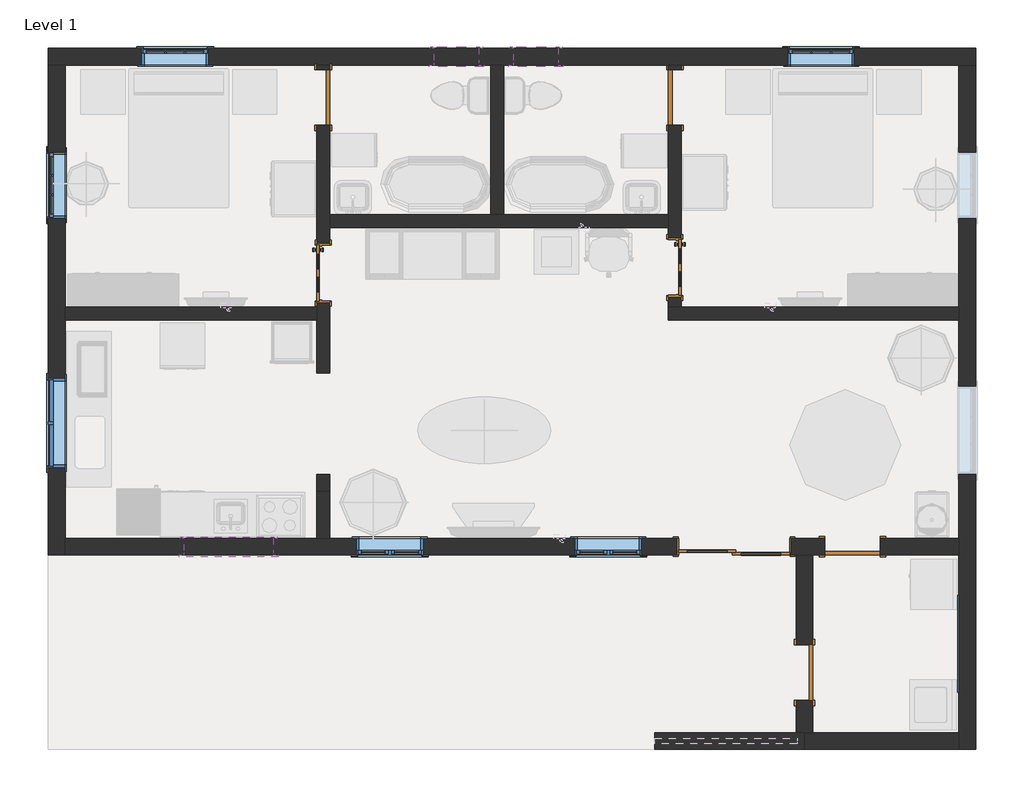
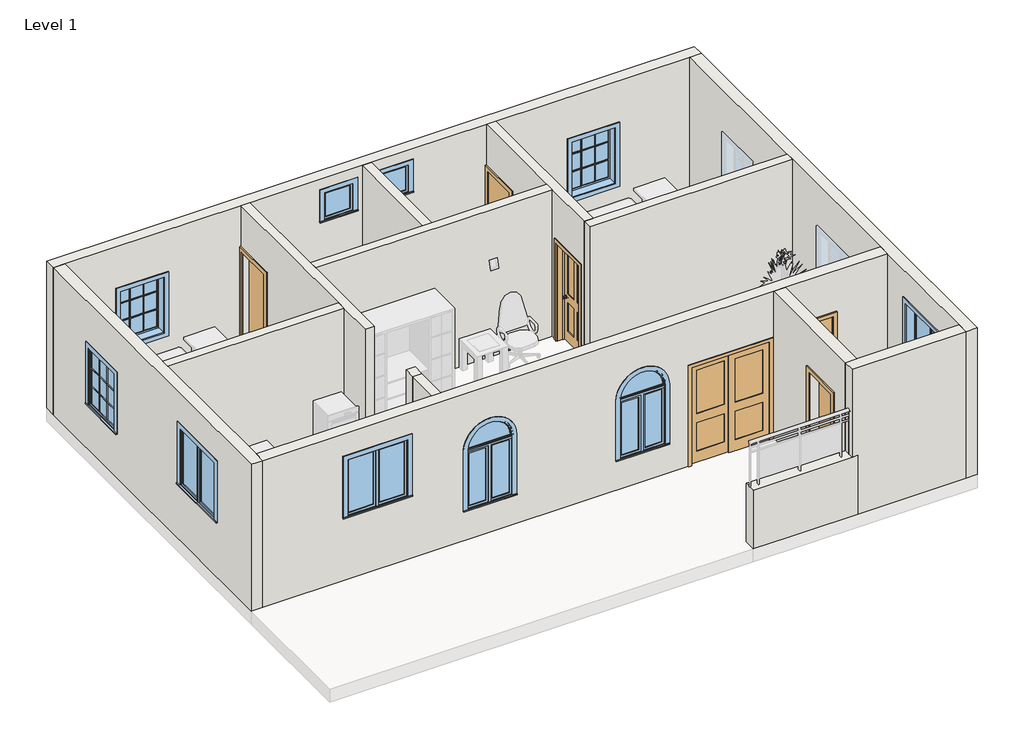
# One storey, part 1 of 2: 15 walls, 10 windows, 7 doors.
"""IFC4 building model written with IfcOpenShell, lengths in millimetres."""

from ifc_helpers import new_model, si_unit, frame, origin, origin_with_axes, place, context, project, spatial, polyline, circle_curve, outline, extrude, faceted_brep, transform, mapped, element, save
from ifc_brep_helpers import plane_surface, revolved_surface, advanced_brep
from components import door_61c74ce0, door_86658926, door_b97b09b3, door_b1104dde, door_0af0cdd0, door_bb98abfd, window_ae0d0e3f, window_642cfea4, window_534dcd48, window_3ed046d9

model = new_model("IFC4")

# Units and contexts
model_context = context("Model", 3, world=origin())
ifc_project = project(units=[si_unit("LENGTHUNIT", "METRE", prefix="MILLI")], contexts=[model_context])

# Site, building, storey
site = spatial("IfcSite", under=ifc_project)
building = spatial("IfcBuilding", under=site)
storey = spatial("IfcBuildingStorey", under=building, Name="Level 1", Elevation=0.0)

# Doors
placement = place(None, origin())
door_shape = door_61c74ce0(model_context)
element("IfcDoor", 1, ObjectType="Door-Interior-Double-Sliding-2_Panel-Wood : 60\" x 80\"", at=placement, inside=storey, context=model_context, shape_type="MappedRepresentation", body=[
    mapped(door_shape, transform((-1370.6447551, 6722.1799175, 0.0), x_axis=(-1.0, 0.0, 0.0), y_axis=(0.0, -1.0, 0.0), z_axis=(0.0, 0.0, 1.0))),
])
door_2_shape = door_86658926(model_context)
element("IfcDoor", 2, ObjectType="Door-Interior-Single-4_Panel-Wood : 30\" x 80\"", at=placement, inside=storey, context=model_context, shape_type="MappedRepresentation", body=[
    mapped(door_2_shape, transform((-7012.6197551, 10484.5549175, 0.0), x_axis=(0.0, -1.0, 0.0), y_axis=(1.0, 0.0, 0.0), z_axis=(0.0, 0.0, 1.0))),
])
door_3_shape = door_b97b09b3(model_context)
element("IfcDoor", 3, ObjectType="Door-Interior-Single-4_Panel-Wood : 30\" x 80\"", at=placement, inside=storey, context=model_context, shape_type="MappedRepresentation", body=[
    mapped(door_3_shape, transform((-2180.2697551, 10560.7549175, 0.0), x_axis=(0.0, -1.0, 0.0), y_axis=(1.0, 0.0, 0.0), z_axis=(0.0, 0.0, 1.0))),
])
door_4_shape = door_b1104dde(model_context)
element("IfcDoor", 4, ObjectType="Single-Flush : 30\" x 84\"", at=placement, inside=storey, context=model_context, shape_type="MappedRepresentation", body=[
    mapped(door_4_shape, transform((-7009.4447551, 12897.5549175, 0.0), x_axis=(0.0, 1.0, 0.0), y_axis=(-1.0, 0.0, 0.0), z_axis=(0.0, 0.0, 1.0))),
])
door_5_shape = door_0af0cdd0(model_context)
element("IfcDoor", 5, ObjectType="Single-Flush : 30\" x 84\"", at=placement, inside=storey, context=model_context, shape_type="MappedRepresentation", body=[
    mapped(door_5_shape, transform((-2183.4447551, 12897.5549175, 0.0), x_axis=(0.0, 1.0, 0.0), y_axis=(-1.0, 0.0, 0.0), z_axis=(0.0, 0.0, 1.0))),
])
door_6_shape = door_bb98abfd(model_context)
element("IfcDoor", 6, ObjectType="Single-Flush : 30\" x 84\"", at=placement, inside=storey, context=model_context, shape_type="MappedRepresentation", body=[
    mapped(door_6_shape, transform((254.9552449, 6725.3549175, 0.0), x_axis=(-1.0, 0.0, 0.0), y_axis=(0.0, -1.0, 0.0), z_axis=(0.0, 0.0, 1.0))),
])
element("IfcDoor", 7, ObjectType="Single-Flush : 30\" x 84\"", at=placement, inside=storey, context=model_context, shape_type="MappedRepresentation", body=[
    mapped(door_6_shape, transform((-405.4447551, 4998.1549175, 0.0), x_axis=(0.0, -1.0, 0.0), y_axis=(1.0, 0.0, 0.0), z_axis=(0.0, 0.0, 1.0))),
])

# Walls
element("IfcWall", 8, ObjectType="Generic - 8\"", at=placement, inside=storey, context=model_context, shape_type="Brep", body=[
    faceted_brep([(-10781.3447551, 13342.0549175, 0.0), (-10552.7447551, 13342.0549175, 0.0), (-7098.3447551, 13342.0549175, 0.0), (-6920.5447551, 13342.0549175, 0.0), (-4710.7447551, 13342.0549175, 0.0), (-4532.9447551, 13342.0549175, 0.0), (-2272.3447551, 13342.0549175, 0.0), (-2094.5447551, 13342.0549175, 0.0), (1715.4552449, 13342.0549175, 0.0), (1944.0552449, 13342.0549175, 0.0), (1944.0552449, 13342.0549175, 3048.0), (1715.4552449, 13342.0549175, 3048.0), (-2094.5447551, 13342.0549175, 3048.0), (-2272.3447551, 13342.0549175, 3048.0), (-4532.9447551, 13342.0549175, 3048.0), (-4710.7447551, 13342.0549175, 3048.0), (-6920.5447551, 13342.0549175, 3048.0), (-7098.3447551, 13342.0549175, 3048.0), (-10552.7447551, 13342.0549175, 3048.0), (-10781.3447551, 13342.0549175, 3048.0), (-8584.2447551, 13342.0549175, 2133.6), (-8584.2447551, 13342.0549175, 914.4), (-9498.6447551, 13342.0549175, 914.4), (-9498.6447551, 13342.0549175, 2133.6), (280.3552449, 13342.0549175, 2133.6), (280.3552449, 13342.0549175, 914.4), (-634.0447551, 13342.0549175, 914.4), (-634.0447551, 13342.0549175, 2133.6), (-5485.4447551, 13342.0549175, 2768.6), (-4875.8447551, 13342.0549175, 2768.6), (-4875.8447551, 13342.0549175, 2159.0), (-5485.4447551, 13342.0549175, 2159.0), (-4393.2447551, 13342.0549175, 2768.6), (-3783.6447551, 13342.0549175, 2768.6), (-3783.6447551, 13342.0549175, 2159.0), (-4393.2447551, 13342.0549175, 2159.0), (-10781.3447551, 13570.6549175, 0.0), (-10781.3447551, 13570.6549175, 3048.0), (1944.0552449, 13570.6549175, 3048.0), (1944.0552449, 13570.6549175, 0.0), (-8584.2447551, 13570.6549175, 2133.6), (-9498.6447551, 13570.6549175, 2133.6), (-9498.6447551, 13570.6549175, 914.4), (-8584.2447551, 13570.6549175, 914.4), (280.3552449, 13570.6549175, 2133.6), (-634.0447551, 13570.6549175, 2133.6), (-634.0447551, 13570.6549175, 914.4), (280.3552449, 13570.6549175, 914.4), (-5485.4447551, 13570.6549175, 2768.6), (-5485.4447551, 13570.6549175, 2159.0), (-4875.8447551, 13570.6549175, 2159.0), (-4875.8447551, 13570.6549175, 2768.6), (-4393.2447551, 13570.6549175, 2768.6), (-4393.2447551, 13570.6549175, 2159.0), (-3783.6447551, 13570.6549175, 2159.0), (-3783.6447551, 13570.6549175, 2768.6)], [[[0, 1, 2, 3, 4, 5, 6, 7, 8, 9, 10, 11, 12, 13, 14, 15, 16, 17, 18, 19], [20, 21, 22, 23], [24, 25, 26, 27], [28, 29, 30, 31], [32, 33, 34, 35]], [[36, 37, 38, 39], [40, 41, 42, 43], [44, 45, 46, 47], [48, 49, 50, 51], [52, 53, 54, 55]], [[9, 8, 7, 6, 5, 4, 3, 2, 1, 0, 36, 39]], [[10, 9, 39, 38]], [[0, 19, 37, 36]], [[19, 18, 17, 16, 15, 14, 13, 12, 11, 10, 38, 37]], [[21, 20, 40, 43]], [[22, 21, 43, 42]], [[23, 22, 42, 41]], [[20, 23, 41, 40]], [[25, 24, 44, 47]], [[26, 25, 47, 46]], [[27, 26, 46, 45]], [[24, 27, 45, 44]], [[49, 48, 28, 31]], [[50, 49, 31, 30]], [[51, 50, 30, 29]], [[48, 51, 29, 28]], [[53, 52, 32, 35]], [[54, 53, 35, 34]], [[55, 54, 34, 33]], [[52, 55, 33, 32]]]),
])
element("IfcWall", 9, ObjectType="Generic - 8\"", at=placement, inside=storey, context=model_context, shape_type="Brep", body=[
    faceted_brep([(1715.4552449, 13342.0549175, 0.0), (1715.4552449, 10014.6549175, 0.0), (1715.4552449, 9836.8549175, 0.0), (1715.4552449, 6839.6549175, 0.0), (1715.4552449, 6611.0549175, 0.0), (1715.4552449, 4172.6549175, 0.0), (1715.4552449, 3944.0549175, 0.0), (1715.4552449, 3944.0549175, 3048.0), (1715.4552449, 4172.6549175, 3048.0), (1715.4552449, 6611.0549175, 3048.0), (1715.4552449, 6839.6549175, 3048.0), (1715.4552449, 9836.8549175, 3048.0), (1715.4552449, 10014.6549175, 3048.0), (1715.4552449, 13342.0549175, 3048.0), (1715.4552449, 11233.8549175, 2133.6), (1715.4552449, 11233.8549175, 914.4), (1715.4552449, 12148.2549175, 914.4), (1715.4552449, 12148.2549175, 2133.6), (1715.4552449, 4782.2549175, 2438.4), (1715.4552449, 4782.2549175, 1219.2), (1715.4552449, 6001.4549175, 1219.2), (1715.4552449, 6001.4549175, 2438.4), (1715.4552449, 7715.9549175, 2133.6), (1715.4552449, 7715.9549175, 609.6), (1715.4552449, 8935.1549175, 609.6), (1715.4552449, 8935.1549175, 2133.6), (1944.0552449, 13342.0549175, 0.0), (1944.0552449, 13342.0549175, 3048.0), (1944.0552449, 3944.0549175, 3048.0), (1944.0552449, 3944.0549175, 0.0), (1944.0552449, 11233.8549175, 2133.6), (1944.0552449, 12148.2549175, 2133.6), (1944.0552449, 12148.2549175, 914.4), (1944.0552449, 11233.8549175, 914.4), (1944.0552449, 4782.2549175, 2438.4), (1944.0552449, 6001.4549175, 2438.4), (1944.0552449, 6001.4549175, 1219.2), (1944.0552449, 4782.2549175, 1219.2), (1944.0552449, 7715.9549175, 2133.6), (1944.0552449, 8935.1549175, 2133.6), (1944.0552449, 8935.1549175, 609.6), (1944.0552449, 7715.9549175, 609.6)], [[[0, 1, 2, 3, 4, 5, 6, 7, 8, 9, 10, 11, 12, 13], [14, 15, 16, 17], [18, 19, 20, 21], [22, 23, 24, 25]], [[26, 27, 28, 29], [30, 31, 32, 33], [34, 35, 36, 37], [38, 39, 40, 41]], [[6, 5, 4, 3, 2, 1, 0, 26, 29]], [[0, 13, 27, 26]], [[7, 6, 29, 28]], [[13, 12, 11, 10, 9, 8, 7, 28, 27]], [[15, 14, 30, 33]], [[16, 15, 33, 32]], [[17, 16, 32, 31]], [[14, 17, 31, 30]], [[19, 18, 34, 37]], [[20, 19, 37, 36]], [[21, 20, 36, 35]], [[18, 21, 35, 34]], [[23, 22, 38, 41]], [[24, 23, 41, 40]], [[25, 24, 40, 39]], [[22, 25, 39, 38]]]),
])
element("IfcWall", 10, ObjectType="Generic - 8\"", at=placement, inside=storey, context=model_context, shape_type="Brep", body=[
    faceted_brep([(1715.4552449, 4172.6549175, 0.0), (-291.1447551, 4172.6549175, 0.0), (-405.4447551, 4172.6549175, 0.0), (-405.4447551, 4172.6549175, 1219.2), (-519.7447551, 4172.6549175, 1219.2), (-519.7447551, 4172.6549175, 3048.0), (-291.1447551, 4172.6549175, 3048.0), (1715.4552449, 4172.6549175, 3048.0), (1715.4552449, 3944.0549175, 0.0), (1715.4552449, 3944.0549175, 3048.0), (-519.7447551, 3944.0549175, 3048.0), (-519.7447551, 3944.0549175, 1219.2), (-405.4447551, 3944.0549175, 1219.2), (-405.4447551, 3944.0549175, 0.0)], [[[0, 1, 2, 3, 4, 5, 6, 7]], [[8, 9, 10, 11, 12, 13]], [[2, 1, 0, 8, 13]], [[0, 7, 9, 8]], [[7, 6, 5, 10, 9]], [[3, 2, 13, 12]], [[11, 4, 3, 12]], [[5, 4, 11, 10]]]),
])
element("IfcWall", 11, ObjectType="Generic - 8\"", at=placement, inside=storey, context=model_context, shape_type="AdvancedBrep", body=[
    advanced_brep(
    [(1715.4552449, 6839.6549175, 3048.0), (1715.4552449, 6839.6549175, 0.0), (635.9552449, 6839.6549175, 0.0), (635.9552449, 6839.6549175, 2133.6), (-126.0447551, 6839.6549175, 2133.6), (-126.0447551, 6839.6549175, 0.0), (-583.2447551, 6839.6549175, 0.0), (-583.2447551, 6839.6549175, 2057.4), (-2158.0447551, 6839.6549175, 2057.4), (-2158.0447551, 6839.6549175, 0.0), (-6920.5447551, 6839.6549175, 0.0), (-7098.3447551, 6839.6549175, 0.0), (-10552.7447551, 6839.6549175, 0.0), (-10552.7447551, 6839.6549175, 3048.0), (-7098.3447551, 6839.6549175, 3048.0), (-6920.5447551, 6839.6549175, 3048.0), (-8914.4447551, 6839.6549175, 2514.6), (-8914.4447551, 6839.6549175, 1295.4), (-7695.2447551, 6839.6549175, 1295.4), (-7695.2447551, 6839.6549175, 2514.6), (-6552.2447551, 6839.6549175, 1847.85), (-6552.2447551, 6839.6549175, 609.6), (-5637.8447551, 6839.6549175, 609.6), (-5637.8447551, 6839.6549175, 1847.85), (-3555.0447551, 6839.6549175, 1847.85), (-3555.0447551, 6839.6549175, 609.6), (-2640.6447551, 6839.6549175, 609.6), (-2640.6447551, 6839.6549175, 1847.85), (1715.4552449, 6611.0549175, 0.0), (1715.4552449, 6611.0549175, 3048.0), (-291.1447551, 6611.0549175, 3048.0), (-519.7447551, 6611.0549175, 3048.0), (-10552.7447551, 6611.0549175, 3048.0), (-10552.7447551, 6611.0549175, 0.0), (-2158.0447551, 6611.0549175, 0.0), (-2158.0447551, 6611.0549175, 2057.4), (-583.2447551, 6611.0549175, 2057.4), (-583.2447551, 6611.0549175, 0.0), (-519.7447551, 6611.0549175, 0.0), (-291.1447551, 6611.0549175, 0.0), (-126.0447551, 6611.0549175, 0.0), (-126.0447551, 6611.0549175, 2133.6), (635.9552449, 6611.0549175, 2133.6), (635.9552449, 6611.0549175, 0.0), (-8914.4447551, 6611.0549175, 2514.6), (-7695.2447551, 6611.0549175, 2514.6), (-7695.2447551, 6611.0549175, 1295.4), (-8914.4447551, 6611.0549175, 1295.4), (-6552.2447551, 6611.0549175, 1847.85), (-5637.8447551, 6611.0549175, 1847.85), (-5637.8447551, 6611.0549175, 609.6), (-6552.2447551, 6611.0549175, 609.6), (-3555.0447551, 6611.0549175, 1847.85), (-2640.6447551, 6611.0549175, 1847.85), (-2640.6447551, 6611.0549175, 609.6), (-3555.0447551, 6611.0549175, 609.6)],
    [
        (0, 1),
        (1, 2),
        (2, 3),
        (3, 4),
        (4, 5),
        (5, 6),
        (6, 7),
        (7, 8),
        (8, 9),
        (9, 10),
        (10, 11),
        (11, 12),
        (12, 13),
        (13, 14),
        (14, 15),
        (15, 0),
        (16, 17),
        (17, 18),
        (18, 19),
        (19, 16),
        (20, 21),
        (21, 22),
        (22, 23),
        (23, 20, circle_curve(frame((-6095.0447551, 6839.6549175, 1847.85), z_axis=(0.0, -1.0, 0.0), x_axis=(-1.0, 0.0, 0.0)), 457.2)),
        (24, 25),
        (25, 26),
        (26, 27),
        (27, 24, circle_curve(frame((-3097.8447551, 6839.6549175, 1847.85), z_axis=(0.0, -1.0, 0.0), x_axis=(-1.0, 0.0, 0.0)), 457.2)),
        (28, 29),
        (29, 30),
        (30, 31),
        (31, 32),
        (32, 33),
        (33, 34),
        (34, 35),
        (35, 36),
        (36, 37),
        (37, 38),
        (38, 39),
        (39, 40),
        (40, 41),
        (41, 42),
        (42, 43),
        (43, 28),
        (44, 45),
        (45, 46),
        (46, 47),
        (47, 44),
        (48, 49, circle_curve(frame((-6095.0447551, 6611.0549175, 1847.85), z_axis=(0.0, 1.0, 0.0), x_axis=(-1.0, 0.0, 0.0)), 457.2)),
        (49, 50),
        (50, 51),
        (51, 48),
        (52, 53, circle_curve(frame((-3097.8447551, 6611.0549175, 1847.85), z_axis=(0.0, 1.0, 0.0), x_axis=(-1.0, 0.0, 0.0)), 457.2)),
        (53, 54),
        (54, 55),
        (55, 52),
        (1, 28),
        (43, 2),
        (33, 12),
        (9, 34),
        (5, 40),
        (37, 6),
        (0, 29),
        (32, 13),
        (4, 41),
        (3, 42),
        (8, 35),
        (7, 36),
        (16, 44),
        (47, 17),
        (46, 18),
        (45, 19),
        (20, 48),
        (51, 21),
        (50, 22),
        (49, 23),
        (24, 52),
        (55, 25),
        (54, 26),
        (53, 27),
    ],
    [
        plane_surface(frame((1829.7552449, 6839.6549175, 0.0), z_axis=(0.0, 1.0, 0.0), x_axis=(-1.0, 0.0, 0.0))),
        plane_surface(frame((1829.7552449, 6611.0549175, 0.0), z_axis=(0.0, -1.0, 0.0), x_axis=(1.0, 0.0, 0.0))),
        plane_surface(frame((1829.7552449, 6839.6549175, 0.0), z_axis=(0.0, 0.0, -1.0), x_axis=(0.0, -1.0, 0.0))),
        plane_surface(frame((1715.4552449, 13456.3549175, 0.0), z_axis=(1.0, 0.0, 0.0), x_axis=(0.0, -1.0, 0.0))),
        plane_surface(frame((-10552.7447551, 4058.3549175, 0.0), z_axis=(-1.0, 0.0, 0.0), x_axis=(0.0, 1.0, 0.0))),
        plane_surface(frame((-10781.3447551, 13570.6549175, 3048.0), z_axis=(0.0, 0.0, 1.0), x_axis=(1.0, 0.0, 0.0))),
        plane_surface(frame((-126.0447551, 6611.0549175, 0.0), z_axis=(1.0, 0.0, 0.0), x_axis=(0.0, 1.0, 0.0))),
        plane_surface(frame((-126.0447551, 6611.0549175, 2133.6), z_axis=(0.0, 0.0, -1.0), x_axis=(0.0, 1.0, 0.0))),
        plane_surface(frame((635.9552449, 6611.0549175, 2133.6), z_axis=(-1.0, 0.0, 0.0), x_axis=(0.0, 1.0, 0.0))),
        plane_surface(frame((-2158.0447551, 8363.6549175, 0.0), z_axis=(1.0, 0.0, 0.0), x_axis=(0.0, -1.0, 0.0))),
        plane_surface(frame((-2158.0447551, 8363.6549175, 2057.4), z_axis=(0.0, 0.0, -1.0), x_axis=(0.0, -1.0, 0.0))),
        plane_surface(frame((-583.2447551, 8363.6549175, 2057.4), z_axis=(-1.0, 0.0, 0.0), x_axis=(0.0, -1.0, 0.0))),
        plane_surface(frame((-8914.4447551, 6839.6549175, 2514.6), z_axis=(1.0, 0.0, 0.0), x_axis=(0.0, -1.0, 0.0))),
        plane_surface(frame((-8914.4447551, 6839.6549175, 1295.4), z_axis=(0.0, 0.0, 1.0), x_axis=(0.0, -1.0, 0.0))),
        plane_surface(frame((-7695.2447551, 6839.6549175, 1295.4), z_axis=(-1.0, 0.0, 0.0), x_axis=(0.0, -1.0, 0.0))),
        plane_surface(frame((-7695.2447551, 6839.6549175, 2514.6), z_axis=(0.0, 0.0, -1.0), x_axis=(0.0, -1.0, 0.0))),
        plane_surface(frame((-6552.2447551, 6839.6549175, 1847.85), z_axis=(1.0, 0.0, 0.0), x_axis=(0.0, -1.0, 0.0))),
        plane_surface(frame((-6552.2447551, 6839.6549175, 609.6), z_axis=(0.0, 0.0, 1.0), x_axis=(0.0, -1.0, 0.0))),
        plane_surface(frame((-5637.8447551, 6839.6549175, 609.6), z_axis=(-1.0, 0.0, 0.0), x_axis=(0.0, -1.0, 0.0))),
        revolved_surface(polyline([(-6552.2447551, 6611.0549175, 1847.85), (-6552.2447551, 6839.6549175, 1847.85)]), (-6095.0447551, 6839.6549175, 1847.85), (0.0, -1.0, 0.0)),
        plane_surface(frame((-3555.0447551, 6839.6549175, 1847.85), z_axis=(1.0, 0.0, 0.0), x_axis=(0.0, -1.0, 0.0))),
        plane_surface(frame((-3555.0447551, 6839.6549175, 609.6), z_axis=(0.0, 0.0, 1.0), x_axis=(0.0, -1.0, 0.0))),
        plane_surface(frame((-2640.6447551, 6839.6549175, 609.6), z_axis=(-1.0, 0.0, 0.0), x_axis=(0.0, -1.0, 0.0))),
        revolved_surface(polyline([(-3555.0447550999997, 6611.0549175, 1847.85), (-3555.0447550999997, 6839.6549175, 1847.85)]), (-3097.8447551, 6839.6549175, 1847.85), (0.0, -1.0, 0.0)),
    ],
    [
        (0, [[1, 2, 3, 4, 5, 6, 7, 8, 9, 10, 11, 12, 13, 14, 15, 16], [17, 18, 19, 20], [21, 22, 23, 24], [25, 26, 27, 28]]),
        (1, [[29, 30, 31, 32, 33, 34, 35, 36, 37, 38, 39, 40, 41, 42, 43, 44], [45, 46, 47, 48], [49, 50, 51, 52], [53, 54, 55, 56]]),
        (2, [[57, -44, 58, -2]]),
        (2, [[59, -12, -11, -10, 60, -34]]),
        (2, [[61, -40, -39, -38, 62, -6]]),
        (3, [[-1, 63, -29, -57]]),
        (4, [[-13, -59, -33, 64]]),
        (5, [[-16, -15, -14, -64, -32, -31, -30, -63]]),
        (6, [[-41, -61, -5, 65]]),
        (7, [[-42, -65, -4, 66]]),
        (8, [[-43, -66, -3, -58]]),
        (9, [[67, -35, -60, -9]]),
        (10, [[-67, -8, 68, -36]]),
        (11, [[-68, -7, -62, -37]]),
        (12, [[-17, 69, -48, 70]]),
        (13, [[-18, -70, -47, 71]]),
        (14, [[-19, -71, -46, 72]]),
        (15, [[-20, -72, -45, -69]]),
        (16, [[-21, 73, -52, 74]]),
        (17, [[-22, -74, -51, 75]]),
        (18, [[-23, -75, -50, 76]]),
        (19, [[-24, -76, -49, -73]]),
        (20, [[-25, 77, -56, 78]]),
        (21, [[-26, -78, -55, 79]]),
        (22, [[-27, -79, -54, 80]]),
        (23, [[-28, -80, -53, -77]]),
    ],
),
])
element("IfcWall", 12, ObjectType="Generic - 8\"", at=placement, inside=storey, context=model_context, shape_type="Brep", body=[
    faceted_brep([(-519.7447551, 4617.1549175, 2133.6), (-519.7447551, 4617.1549175, 0.0), (-519.7447551, 4172.6549175, 0.0), (-519.7447551, 4172.6549175, 1219.2), (-519.7447551, 4172.6549175, 3048.0), (-519.7447551, 6611.0549175, 3048.0), (-519.7447551, 6611.0549175, 0.0), (-519.7447551, 5379.1549175, 0.0), (-519.7447551, 5379.1549175, 2133.6), (-291.1447551, 4172.6549175, 0.0), (-291.1447551, 4617.1549175, 0.0), (-291.1447551, 4617.1549175, 2133.6), (-291.1447551, 5379.1549175, 2133.6), (-291.1447551, 5379.1549175, 0.0), (-291.1447551, 6611.0549175, 0.0), (-291.1447551, 6611.0549175, 3048.0), (-291.1447551, 4172.6549175, 3048.0), (-405.4447551, 4172.6549175, 0.0)], [[[0, 1, 2, 3, 4, 5, 6, 7, 8]], [[9, 10, 11, 12, 13, 14, 15, 16]], [[7, 6, 14, 13]], [[2, 1, 10, 9, 17]], [[6, 5, 15, 14]], [[5, 4, 16, 15]], [[11, 10, 1, 0]], [[12, 11, 0, 8]], [[13, 12, 8, 7]], [[2, 17, 9, 16, 4, 3]]]),
])
element("IfcWall", 13, ObjectType="Generic - 8\"", at=placement, inside=storey, context=model_context, shape_type="Brep", body=[
    faceted_brep([(-10552.7447551, 6611.0549175, 0.0), (-10552.7447551, 6839.6549175, 0.0), (-10552.7447551, 9836.8549175, 0.0), (-10552.7447551, 10014.6549175, 0.0), (-10552.7447551, 13342.0549175, 0.0), (-10552.7447551, 13342.0549175, 3048.0), (-10552.7447551, 10014.6549175, 3048.0), (-10552.7447551, 9836.8549175, 3048.0), (-10552.7447551, 6839.6549175, 3048.0), (-10552.7447551, 6611.0549175, 3048.0), (-10552.7447551, 12148.2549175, 2133.6), (-10552.7447551, 12148.2549175, 914.4), (-10552.7447551, 11233.8549175, 914.4), (-10552.7447551, 11233.8549175, 2133.6), (-10552.7447551, 9036.7549175, 2362.2), (-10552.7447551, 9036.7549175, 1143.0), (-10552.7447551, 7817.5549175, 1143.0), (-10552.7447551, 7817.5549175, 2362.2), (-10781.3447551, 6611.0549175, 0.0), (-10781.3447551, 6611.0549175, 3048.0), (-10781.3447551, 13342.0549175, 3048.0), (-10781.3447551, 13342.0549175, 0.0), (-10781.3447551, 12148.2549175, 2133.6), (-10781.3447551, 11233.8549175, 2133.6), (-10781.3447551, 11233.8549175, 914.4), (-10781.3447551, 12148.2549175, 914.4), (-10781.3447551, 9036.7549175, 2362.2), (-10781.3447551, 7817.5549175, 2362.2), (-10781.3447551, 7817.5549175, 1143.0), (-10781.3447551, 9036.7549175, 1143.0)], [[[0, 1, 2, 3, 4, 5, 6, 7, 8, 9], [10, 11, 12, 13], [14, 15, 16, 17]], [[18, 19, 20, 21], [22, 23, 24, 25], [26, 27, 28, 29]], [[4, 3, 2, 1, 0, 18, 21]], [[5, 4, 21, 20]], [[0, 9, 19, 18]], [[9, 8, 7, 6, 5, 20, 19]], [[11, 10, 22, 25]], [[12, 11, 25, 24]], [[13, 12, 24, 23]], [[10, 13, 23, 22]], [[15, 14, 26, 29]], [[16, 15, 29, 28]], [[17, 16, 28, 27]], [[14, 17, 27, 26]]]),
])
element("IfcWall", 14, ObjectType="Generic - 8\"", at=placement, inside=storey, context=model_context, shape_type="Brep", body=[
    faceted_brep([(-405.4447551, 4172.6549175, 0.0), (-519.7447551, 4172.6549175, 0.0), (-2462.8447551, 4172.6549175, 0.0), (-2462.8447551, 4172.6549175, 1219.2), (-519.7447551, 4172.6549175, 1219.2), (-405.4447551, 4172.6549175, 1219.2), (-405.4447551, 3944.0549175, 0.0), (-405.4447551, 3944.0549175, 1219.2), (-519.7447551, 3944.0549175, 1219.2), (-2462.8447551, 3944.0549175, 1219.2), (-2462.8447551, 3944.0549175, 0.0)], [[[0, 1, 2, 3, 4, 5]], [[6, 7, 8, 9, 10]], [[2, 1, 0, 6, 10]], [[3, 2, 10, 9]], [[5, 4, 3, 9, 8, 7]], [[0, 5, 7, 6]]]),
])
element("IfcWall", 15, ObjectType="INNER WALL", at=placement, inside=storey, context=model_context, shape_type="Brep", body=[
    faceted_brep([(1715.4552449, 10014.6549175, 0.0), (-2094.5447551, 10014.6549175, 0.0), (-2272.3447551, 10014.6549175, 0.0), (-2272.3447551, 10014.6549175, 3048.0), (-2094.5447551, 10014.6549175, 3048.0), (1715.4552449, 10014.6549175, 3048.0), (1715.4552449, 9836.8549175, 0.0), (1715.4552449, 9836.8549175, 3048.0), (-2272.3447551, 9836.8549175, 3048.0), (-2272.3447551, 9836.8549175, 0.0)], [[[0, 1, 2, 3, 4, 5]], [[6, 7, 8, 9]], [[2, 1, 0, 6, 9]], [[0, 5, 7, 6]], [[3, 2, 9, 8]], [[5, 4, 3, 8, 7]]]),
])
element("IfcWall", 16, ObjectType="INNER WALL", at=placement, inside=storey, context=model_context, shape_type="Brep", body=[
    faceted_brep([(-7098.3447551, 9112.9549175, 0.0), (-7098.3447551, 9112.9549175, 3048.0), (-7098.3447551, 9836.8549175, 3048.0), (-7098.3447551, 10014.6549175, 3048.0), (-7098.3447551, 13342.0549175, 3048.0), (-7098.3447551, 13342.0549175, 0.0), (-7098.3447551, 13278.5549175, 0.0), (-7098.3447551, 13278.5549175, 2133.6), (-7098.3447551, 12516.5549175, 2133.6), (-7098.3447551, 12516.5549175, 0.0), (-7098.3447551, 10890.9549175, 0.0), (-7098.3447551, 10890.9549175, 2057.4), (-7098.3447551, 10078.1549175, 2057.4), (-7098.3447551, 10078.1549175, 0.0), (-7098.3447551, 10014.6549175, 0.0), (-7098.3447551, 9836.8549175, 0.0), (-6920.5447551, 9112.9549175, 3048.0), (-6920.5447551, 9112.9549175, 0.0), (-6920.5447551, 10078.1549175, 0.0), (-6920.5447551, 10078.1549175, 2057.4), (-6920.5447551, 10890.9549175, 2057.4), (-6920.5447551, 10890.9549175, 0.0), (-6920.5447551, 11106.8549175, 0.0), (-6920.5447551, 11284.6549175, 0.0), (-6920.5447551, 12516.5549175, 0.0), (-6920.5447551, 12516.5549175, 2133.6), (-6920.5447551, 13278.5549175, 2133.6), (-6920.5447551, 13278.5549175, 0.0), (-6920.5447551, 13342.0549175, 0.0), (-6920.5447551, 13342.0549175, 3048.0), (-6920.5447551, 11284.6549175, 3048.0), (-6920.5447551, 11106.8549175, 3048.0)], [[[0, 1, 2, 3, 4, 5, 6, 7, 8, 9, 10, 11, 12, 13, 14, 15]], [[16, 17, 18, 19, 20, 21, 22, 23, 24, 25, 26, 27, 28, 29, 30, 31]], [[17, 0, 15, 14, 13, 18]], [[5, 28, 27, 6]], [[9, 24, 23, 22, 21, 10]], [[1, 0, 17, 16]], [[5, 4, 29, 28]], [[4, 3, 2, 1, 16, 31, 30, 29]], [[7, 6, 27, 26]], [[8, 7, 26, 25]], [[9, 8, 25, 24]], [[12, 19, 18, 13]], [[19, 12, 11, 20]], [[20, 11, 10, 21]]]),
])
element("IfcWall", 17, ObjectType="INNER WALL", at=placement, inside=storey, context=model_context, shape_type="Brep", body=[
    faceted_brep([(-2272.3447551, 13342.0549175, 3048.0), (-2272.3447551, 13342.0549175, 0.0), (-2272.3447551, 13278.5549175, 0.0), (-2272.3447551, 13278.5549175, 2133.6), (-2272.3447551, 12516.5549175, 2133.6), (-2272.3447551, 12516.5549175, 0.0), (-2272.3447551, 11284.6549175, 0.0), (-2272.3447551, 11106.8549175, 0.0), (-2272.3447551, 10967.1549175, 0.0), (-2272.3447551, 10967.1549175, 2057.4), (-2272.3447551, 10154.3549175, 2057.4), (-2272.3447551, 10154.3549175, 0.0), (-2272.3447551, 10014.6549175, 0.0), (-2272.3447551, 10014.6549175, 3048.0), (-2272.3447551, 11106.8549175, 3048.0), (-2272.3447551, 11284.6549175, 3048.0), (-2094.5447551, 13342.0549175, 0.0), (-2094.5447551, 13342.0549175, 3048.0), (-2094.5447551, 10014.6549175, 3048.0), (-2094.5447551, 10014.6549175, 0.0), (-2094.5447551, 10154.3549175, 0.0), (-2094.5447551, 10154.3549175, 2057.4), (-2094.5447551, 10967.1549175, 2057.4), (-2094.5447551, 10967.1549175, 0.0), (-2094.5447551, 12516.5549175, 0.0), (-2094.5447551, 12516.5549175, 2133.6), (-2094.5447551, 13278.5549175, 2133.6), (-2094.5447551, 13278.5549175, 0.0)], [[[0, 1, 2, 3, 4, 5, 6, 7, 8, 9, 10, 11, 12, 13, 14, 15]], [[16, 17, 18, 19, 20, 21, 22, 23, 24, 25, 26, 27]], [[1, 16, 27, 2]], [[19, 12, 11, 20]], [[5, 24, 23, 8, 7, 6]], [[1, 0, 17, 16]], [[13, 12, 19, 18]], [[0, 15, 14, 13, 18, 17]], [[3, 2, 27, 26]], [[4, 3, 26, 25]], [[5, 4, 25, 24]], [[10, 21, 20, 11]], [[21, 10, 9, 22]], [[22, 9, 8, 23]]]),
])
element("IfcWall", 18, ObjectType="INNER WALL", at=placement, inside=storey, context=model_context, shape_type="Brep", body=[
    faceted_brep([(-2272.3447551, 11284.6549175, 0.0), (-4532.9447551, 11284.6549175, 0.0), (-4710.7447551, 11284.6549175, 0.0), (-6920.5447551, 11284.6549175, 0.0), (-6920.5447551, 11284.6549175, 3048.0), (-4710.7447551, 11284.6549175, 3048.0), (-4532.9447551, 11284.6549175, 3048.0), (-2272.3447551, 11284.6549175, 3048.0), (-2272.3447551, 11106.8549175, 0.0), (-2272.3447551, 11106.8549175, 3048.0), (-6920.5447551, 11106.8549175, 3048.0), (-6920.5447551, 11106.8549175, 0.0)], [[[0, 1, 2, 3, 4, 5, 6, 7]], [[8, 9, 10, 11]], [[3, 2, 1, 0, 8, 11]], [[4, 3, 11, 10]], [[0, 7, 9, 8]], [[7, 6, 5, 4, 10, 9]]]),
])
element("IfcWall", 19, ObjectType="INNER WALL", at=placement, inside=storey, context=model_context, shape_type="SweptSolid", body=[
    extrude(outline(polyline([(-10552.7447551, 10014.6549175), (-7098.3447551, 10014.6549175), (-7098.3447551, 9836.8549175), (-10552.7447551, 9836.8549175), (-10552.7447551, 10014.6549175)])), origin_with_axes(), (0.0, 0.0, 1.0), 3048.0),
])
element("IfcWall", 20, ObjectType="INNER WALL", at=placement, inside=storey, context=model_context, shape_type="SweptSolid", body=[
    extrude(outline(polyline([(-4532.9447551, 13342.0549175), (-4532.9447551, 11284.6549175), (-4710.7447551, 11284.6549175), (-4710.7447551, 13342.0549175), (-4532.9447551, 13342.0549175)])), origin_with_axes(), (0.0, 0.0, 1.0), 3048.0),
])
element("IfcWall", 21, ObjectType="INNER WALL", at=placement, inside=storey, context=model_context, shape_type="SweptSolid", body=[
    extrude(outline(polyline([(-7098.3447551, 6839.6549175), (-7098.3447551, 7487.3549175), (-6920.5447551, 7487.3549175), (-6920.5447551, 6839.6549175), (-7098.3447551, 6839.6549175)])), origin_with_axes(), (0.0, 0.0, 1.0), 3048.0),
])
element("IfcWall", 22, ObjectType="INNER WALL", at=placement, inside=storey, context=model_context, shape_type="SweptSolid", body=[
    extrude(outline(polyline([(-6920.5447551, 7715.9549175), (-6920.5447551, 7487.3549175), (-7098.3447551, 7487.3549175), (-7098.3447551, 7715.9549175), (-6920.5447551, 7715.9549175)])), origin_with_axes(), (0.0, 0.0, 1.0), 3048.0),
])

# Windows
window_shape = window_ae0d0e3f(model_context)
element("IfcWindow", 23, ObjectType="36\" x 48\"", at=placement, inside=storey, context=model_context, shape_type="MappedRepresentation", body=[
    mapped(window_shape, transform((-6087.042597, 6725.3549175, 304.8), x_axis=(-1.0, 0.0, 0.0), y_axis=(0.0, -1.0, 0.0), z_axis=(0.0, 0.0, 1.0))),
])
element("IfcWindow", 24, ObjectType="36\" x 48\"", at=placement, inside=storey, context=model_context, shape_type="MappedRepresentation", body=[
    mapped(window_shape, transform((-3089.842597, 6725.3549175, 304.8), x_axis=(-1.0, 0.0, 0.0), y_axis=(0.0, -1.0, 0.0), z_axis=(0.0, 0.0, 1.0))),
])
window_2_shape = window_642cfea4(model_context)
element("IfcWindow", 25, ObjectType="Casement 3x3 with Trim : 36\" x 48\"", at=placement, inside=storey, context=model_context, shape_type="MappedRepresentation", body=[
    mapped(window_2_shape, transform((-10667.0447551, 11691.0549175, 304.8), x_axis=(0.0, 1.0, 0.0), y_axis=(-1.0, 0.0, 0.0), z_axis=(0.0, 0.0, 1.0))),
])
element("IfcWindow", 26, ObjectType="Casement 3x3 with Trim : 36\" x 48\"", at=placement, inside=storey, context=model_context, shape_type="MappedRepresentation", body=[
    mapped(window_2_shape, transform((-9041.4447551, 13456.3549175, 304.8), x_axis=(1.0, 0.0, 0.0), y_axis=(0.0, 1.0, 0.0), z_axis=(0.0, 0.0, 1.0))),
])
element("IfcWindow", 27, ObjectType="Casement 3x3 with Trim : 36\" x 48\"", at=placement, inside=storey, context=model_context, shape_type="MappedRepresentation", body=[
    mapped(window_2_shape, transform((-176.8447551, 13456.3549175, 304.8), x_axis=(1.0, 0.0, 0.0), y_axis=(0.0, 1.0, 0.0), z_axis=(0.0, 0.0, 1.0))),
])
window_3_shape = window_534dcd48(model_context)
element("IfcWindow", 28, ObjectType="Casement Dbl with Trim : 48\" x 48\"", at=placement, inside=storey, context=model_context, shape_type="MappedRepresentation", body=[
    mapped(window_3_shape, transform((-10647.9947551, 8427.1549175, 228.6), x_axis=(0.0, 1.0, 0.0), y_axis=(-1.0, 0.0, 0.0), z_axis=(0.0, 0.0, 1.0))),
])
element("IfcWindow", 29, ObjectType="Casement Dbl with Trim : 48\" x 48\"", at=placement, inside=storey, context=model_context, shape_type="MappedRepresentation", body=[
    mapped(window_3_shape, transform((-8304.8447551, 6744.4049175, 381.0), x_axis=(-1.0, 0.0, 0.0), y_axis=(0.0, -1.0, 0.0), z_axis=(0.0, 0.0, 1.0))),
])
element("IfcWindow", 30, ObjectType="Casement Dbl with Trim : 48\" x 48\"", at=placement, inside=storey, context=model_context, shape_type="MappedRepresentation", body=[
    mapped(window_3_shape, transform((1810.7052449, 5391.8549175, 304.8), x_axis=(0.0, -1.0, 0.0), y_axis=(1.0, 0.0, 0.0), z_axis=(0.0, 0.0, 1.0))),
])
window_4_shape = window_3ed046d9(model_context)
element("IfcWindow", 31, ObjectType="Transom with Trim : 24\" x 24\"", at=placement, inside=storey, context=model_context, shape_type="MappedRepresentation", body=[
    mapped(window_4_shape, transform((-5218.7447551, 13456.3549175, 0.0), x_axis=(-1.0, 0.0, 0.0), y_axis=(0.0, -1.0, 0.0), z_axis=(0.0, 0.0, 1.0))),
])
element("IfcWindow", 32, ObjectType="Transom with Trim : 24\" x 24\"", at=placement, inside=storey, context=model_context, shape_type="MappedRepresentation", body=[
    mapped(window_4_shape, transform((-4126.5447551, 13456.3549175, 0.0), x_axis=(-1.0, 0.0, 0.0), y_axis=(0.0, -1.0, 0.0), z_axis=(0.0, 0.0, 1.0))),
])

save(model, "model.ifc")

# Revit data of these elements
# Type "Door-Interior-Double-Sliding-2_Panel-Wood : 60\" x 80\""
#   Type Mark = "8"
#   Assembly Code = "C1020300"
#   Analytic Construction = "Wooden"
#   Top Rail = 0' - 4 11/16"
#   Thickness = 0' - 1 3/8"
#   Thermal Resistance (R) = 2.5876 (h·ft²·°F)/BTU
#   Stiles = 0' - 4 3/4"
#   Rough Width = 5' - 2"
#   Rough Height = 6' - 9"
#   Lock Rail = 0' - 7 1/2"
#   Height = 6' - 8"
#   Width = 5' - 0"
#   Heat Transfer Coefficient (U) = 0.3865 BTU/(h·ft²·°F)
#   Bottom Rail = 0' - 9 1/8"
#   Trim Material = Cherry
#   Panel Material = Cherry
#   Frame Material = Cherry
#   Visual Light Transmittance = 0
#   Solar Heat Gain Coefficient = 0
#   Wall Closure = (empty or 0)
#   Function = (empty or 0)
# Type "Door-Interior-Single-4_Panel-Wood : 30\" x 80\""
#   Type Mark = "9"
#   Assembly Code = "C1020300"
#   Analytic Construction = "Wooden"
#   Top Rail = 0' - 4 11/16"
#   Thickness = 0' - 1 3/8"
#   Thermal Resistance (R) = 2.5876 (h·ft²·°F)/BTU
#   Swing Angle [instance default] = 90.00°
#   Stiles = 0' - 4 3/4"
#   Rough Width = 2' - 8"
#   Rough Height = 6' - 9"
#   Mullion = 0' - 4 1/2"
#   Lock Rail = 0' - 7 1/2"
#   Height = 6' - 8"
#   Width = 2' - 6"
#   Heat Transfer Coefficient (U) = 0.3865 BTU/(h·ft²·°F)
#   Bottom Rail = 0' - 9 1/8"
#   Trim Material = Cherry
#   Panel Material = Cherry
#   Frame Material = Cherry
#   Door Handle Material = Aluminum
#   Visual Light Transmittance = 0
#   Solar Heat Gain Coefficient = 0
#   Wall Closure = (empty or 0)
#   Function = (empty or 0)
# Type "Single-Flush : 30\" x 84\""
#   Type Mark = "4"
#   Construction Type Id = "MDOOR"
#   Assembly Code = "C1020"
#   Analytic Construction = "Metal"
#   Thickness = 0' - 2"
#   Heat Transfer Coefficient (U) = 0.651978 BTU/(h·ft²·°F)
#   Height = 7' - 0"
#   Trim Projection Ext = 0' - 1"
#   Trim Projection Int = 0' - 1"
#   Trim Width = 0' - 3"
#   Width = 2' - 6"
#   Define Thermal Properties by = 1
#   Door Material = Door - Panel
#   Frame Material = Door - Frame
#   Visual Light Transmittance = 0
#   Solar Heat Gain Coefficient = 0
#   Function = (empty or 0)
#   Wall Closure = (empty or 0)
# Type "Generic - 8\""
#   Assembly Code = "B2010"
#   Layers, outside or top first: 0' - 9" "Asphalt Shingle" (function 1)
# Type "INNER WALL"
#   Assembly Code = "B2010"
#   Layers, outside or top first: 0' - 7" "Asphalt Shingle" (function 1)
# Type "36\" x 48\""
#   Type Mark = "16"
#   Construction Type Id = "SGL"
#   Assembly Code = "B2020100"
#   Analytic Construction = "Large single-glazed windows"
#   Visual Light Transmittance = 0.9
#   Solar Heat Gain Coefficient = 0.86
#   Heat Transfer Coefficient (U) = 0.979472 BTU/(h·ft²·°F)
#   Height = 4' - 0"
#   Default Sill Height = 1' - 0"
#   Trim Projection - Ext. = 0' - 0 1/2"
#   Trim Projection - Int. = 0' - 0 3/4"
#   Trim Width - Exterior = 0' - 3 1/2"
#   Trim Width - Interior = 0' - 3 1/2"
#   Width = 3' - 0"
#   Window Inset = 0' - 0 3/4"
#   Define Thermal Properties by = 1
#   Glass Pane Material = Glass
#   Sash Material = Sash
#   Trim Exterior Material = Trim
#   Trim Interior Material = Trim
#   Wall Closure = (empty or 0)
# Type "Casement 3x3 with Trim : 36\" x 48\""
#   Type Mark = "11"
#   Construction Type Id = "GSP4R"
#   Assembly Code = "B2020100"
#   Analytic Construction = "1/8 in Pilkington single glazing"
#   Visual Light Transmittance = 0.9
#   Solar Heat Gain Coefficient = 0.78
#   Heat Transfer Coefficient (U) = 0.6496 BTU/(h·ft²·°F)
#   Height = 4' - 0"
#   Default Sill Height = 2' - 0"
#   Trim Projection - Ext. = 0' - 0 1/2"
#   Trim Projection - Int. = 0' - 0 3/4"
#   Trim Width - Exterior = 0' - 3 1/2"
#   Trim Width - Interior = 0' - 3 1/2"
#   Width = 3' - 0"
#   Window Inset = 0' - 0 3/4"
#   Define Thermal Properties by = 1
#   Glass Pane Material = Glass
#   Sash Material = Softwood, Lumber
#   Trim Exterior Material = Trim
#   Trim Interior Material = Trim
#   Wall Closure = (empty or 0)
# Type "Casement Dbl with Trim : 48\" x 48\""
#   Type Mark = "13"
#   Construction Type Id = "GSP4R"
#   Assembly Code = "B2020100"
#   Analytic Construction = "1/8 in Pilkington single glazing"
#   Visual Light Transmittance = 0.9
#   Solar Heat Gain Coefficient = 0.78
#   Heat Transfer Coefficient (U) = 0.6496 BTU/(h·ft²·°F)
#   Height = 4' - 0"
#   Default Sill Height = 3' - 0"
#   Trim Projection - Ext. = 0' - 0 1/2"
#   Trim Projection - Int. = 0' - 0 3/4"
#   Trim Width - Exterior = 0' - 3 1/2"
#   Trim Width - Interior = 0' - 3 1/2"
#   Width = 4' - 0"
#   Window Inset = 0' - 0 3/4"
#   Define Thermal Properties by = 1
#   Glass Pane Material = Glass
#   Sash Material = Sash
#   Trim Exterior Material = Trim
#   Trim Interior Material = Trim
#   Wall Closure = (empty or 0)
# Type "Transom with Trim : 24\" x 24\""
#   Type Mark = "20"
#   Construction Type Id = "GSP4R"
#   Assembly Code = "B2020100"
#   Analytic Construction = "1/8 in Pilkington single glazing"
#   Visual Light Transmittance = 0.9
#   Solar Heat Gain Coefficient = 0.78
#   Heat Transfer Coefficient (U) = 0.6496 BTU/(h·ft²·°F)
#   Height = 2' - 0"
#   Default Sill Height = 7' - 1"
#   Trim Projection - Ext. = 0' - 0 1/2"
#   Trim Projection - Int. = 0' - 0 3/4"
#   Trim Width - Exterior = 0' - 3 1/2"
#   Trim Width - Interior = 0' - 3 1/2"
#   Width = 2' - 0"
#   Window Inset = 0' - 0 3/4"
#   Define Thermal Properties by = 1
#   Glass Pane Material = Glass
#   Sash Material = Sash
#   Trim Exterior Material = Trim
#   Trim Interior Material = Trim
#   Wall Closure = (empty or 0)
# Element 1 (IfcDoor, "Door-Interior-Double-Sliding-2_Panel-Wood : 60\" x 80\"")
#   Phase Created = New Construction
#   Materials on its faces: "Cherry"
# Elements 2, 3 (IfcDoor, "Door-Interior-Single-4_Panel-Wood : 30\" x 80\"")
#   Swing Angle = 90.00°
#   Phase Created = New Construction
#   Materials on its faces: "Cherry", "Aluminum"
# Elements 4, 5, 6, 7 (IfcDoor, "Single-Flush : 30\" x 84\"")
#   Phase Created = New Construction
#   Materials on its faces: "Door - Frame", "Door - Panel"
# Elements 8, 9, 10, 11, 12, 13 (IfcWall, "Generic - 8\"")
#   Top Offset = 0' - 0"
#   Base Offset = 0' - 0"
#   Unconnected Height = 10' - 0"
#   wall height = 10' - 0"
#   Phase Created = New Construction
#   Base Constraint = Level 1
#   Materials on its faces: "Asphalt Shingle"
# Element 14 (IfcWall, "Generic - 8\"")
#   Top Offset = 0' - 0"
#   Base Offset = 0' - 0"
#   Unconnected Height = 4' - 0"
#   wall height = 4' - 0"
#   Phase Created = New Construction
#   Base Constraint = Level 1
#   Materials on its faces: "Asphalt Shingle"
# Elements 15, 16, 17, 18, 19, 20, 21, 22 (IfcWall, "INNER WALL")
#   Top Offset = 0' - 0"
#   Base Offset = 0' - 0"
#   Unconnected Height = 10' - 0"
#   wall height = 10' - 0"
#   Phase Created = New Construction
#   Base Constraint = Level 1
#   Materials on its faces: "Asphalt Shingle"
# Element 23 (IfcWindow, "36\" x 48\"")
#   Mark = "9"
#   Phase Created = New Construction
#   Materials on its faces: "Sash", "Trim", "Glass"
# Element 24 (IfcWindow, "36\" x 48\"")
#   Mark = "10"
#   Phase Created = New Construction
#   Materials on its faces: "Sash", "Trim", "Glass"
# Element 25 (IfcWindow, "Casement 3x3 with Trim : 36\" x 48\"")
#   Mark = "1"
#   Phase Created = New Construction
#   Materials on its faces: "Softwood, Lumber", "Glass", "Trim"
# Element 26 (IfcWindow, "Casement 3x3 with Trim : 36\" x 48\"")
#   Mark = "2"
#   Phase Created = New Construction
#   Materials on its faces: "Softwood, Lumber", "Glass", "Trim"
# Element 27 (IfcWindow, "Casement 3x3 with Trim : 36\" x 48\"")
#   Mark = "3"
#   Phase Created = New Construction
#   Materials on its faces: "Softwood, Lumber", "Glass", "Trim"
# Element 28 (IfcWindow, "Casement Dbl with Trim : 48\" x 48\"")
#   Mark = "5"
#   Phase Created = New Construction
#   Materials on its faces: "Sash", "Trim", "Glass"
# Element 29 (IfcWindow, "Casement Dbl with Trim : 48\" x 48\"")
#   Mark = "6"
#   Phase Created = New Construction
#   Materials on its faces: "Sash", "Trim", "Glass"
# Element 30 (IfcWindow, "Casement Dbl with Trim : 48\" x 48\"")
#   Mark = "7"
#   Phase Created = New Construction
#   Materials on its faces: "Sash", "Trim", "Glass"
# Element 31 (IfcWindow, "Transom with Trim : 24\" x 24\"")
#   Mark = "11"
#   Phase Created = New Construction
#   Materials on its faces: "Sash", "Trim", "Glass"
# Element 32 (IfcWindow, "Transom with Trim : 24\" x 24\"")
#   Mark = "12"
#   Phase Created = New Construction
#   Materials on its faces: "Sash", "Trim", "Glass"
# Materials
#   "Cherry": class "Wood", colour RGB 226 177 128, transparency 0, Description = "Prunus Serotina", Cost = 0
#   "Aluminum": class "Metal", colour RGB 247 247 247, transparency 0, Description = "Aluminum 6061", Cost = 0
#   "Door - Panel": class "Wood", colour RGB 210 159 95, transparency 0
#   "Door - Frame": colour RGB 118 70 51, transparency 0
#   "Asphalt Shingle": class "Generic", colour RGB 155 155 155, transparency 0, Description = "Asphalt roofing shingle", Cost = 0
#   "Glass": class "Glass", colour RGB 0 128 192, transparency 0.75, Description = "Soda Lime Glass", Cost = 0
#   "Sash": class "Wood", colour RGB 224 178 126, transparency 0
#   "Trim": class "Wood", colour RGB 224 178 126, transparency 0
#   "Softwood, Lumber": class "Wood", colour RGB 223 192 134, transparency 0, Description = "Pinus Echinata", Cost = 0
# Room at (-1431.847, 5378.877) mm, phase "New Construction", upper level "Level 1", upper offset 10' - 0", lower offset 0' - 0"
#   Number = "1"
#   Name = "PORCH"
# Room at (648.276, 5378.877) mm, phase "New Construction", upper level "Level 1", upper offset 10' - 0", lower offset 0' - 0"
#   Number = "2"
#   Name = "Laundry"
# Room at (0, 12002.428) mm, phase "New Construction", upper level "Level 1", upper offset 10' - 0", lower offset 0' - 0"
#   Number = "3"
#   Name = "BEDROOM"
# Room at (-9204.94, 11746.974) mm, phase "New Construction", upper level "Level 1", upper offset 10' - 0", lower offset 0' - 0"
#   Number = "4"
#   Name = "BEDROOM"
# Room at (-5738.068, 12422.102) mm, phase "New Construction", upper level "Level 1", upper offset 10' - 0", lower offset 0' - 0"
#   Number = "5"
#   Name = "Bathroom"
# Room at (-3530.217, 12422.102) mm, phase "New Construction", upper level "Level 1", upper offset 10' - 0", lower offset 0' - 0"
#   Number = "6"
#   Name = "Bathroom"
# Room at (-8931.24, 8462.569) mm, phase "New Construction", upper level "Level 1", upper offset 10' - 0", lower offset 0' - 0"
#   Number = "7"
#   Name = "KITCHEN"
# Room at (0, 8462.569) mm, phase "New Construction", upper level "Level 1", upper offset 10' - 0", lower offset 0' - 0"
#   Number = "8"
#   Name = "DINING ROOM"
# Room at (-4515.539, 9724.724) mm, phase "New Construction", upper level "Level 1", upper offset 10' - 0", lower offset 0' - 0"
#   Number = "9"
#   Name = "LIVING ROOM"
